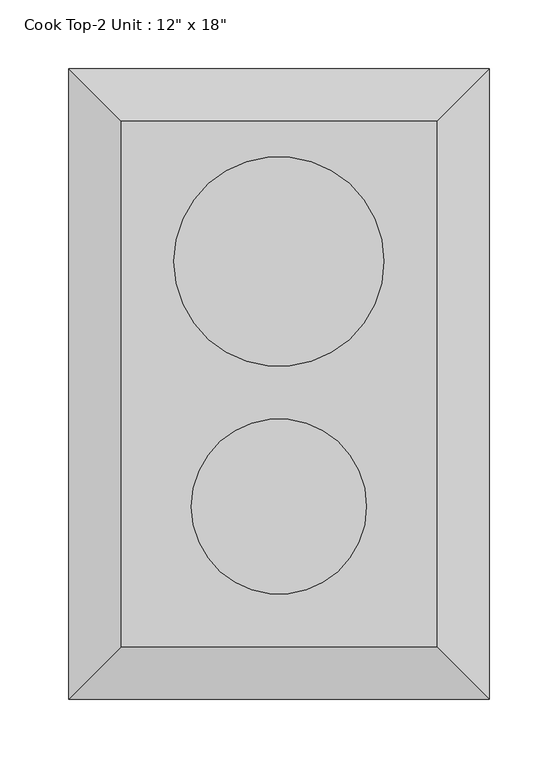
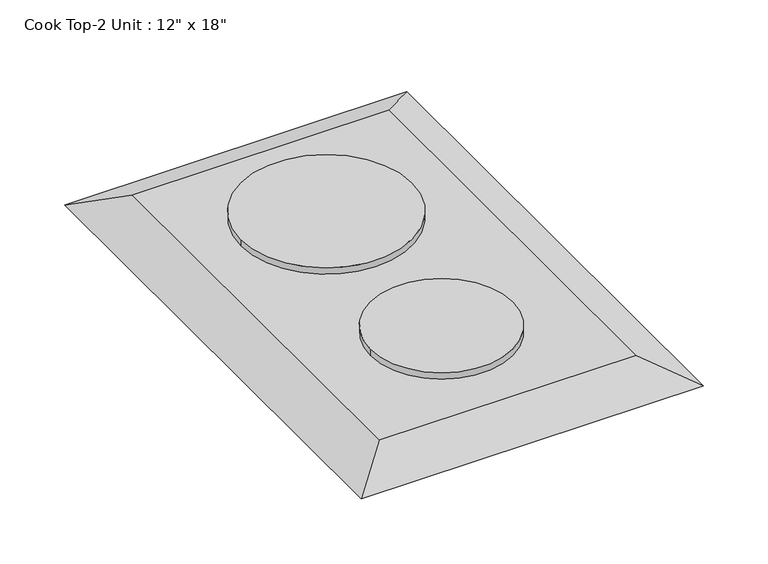
"""IFC4 building model written with IfcOpenShell, lengths in millimetres: proxy geometry."""

from ifc_helpers import new_model, si_unit, point, frame, frame_2d, origin, place, context, project, spatial, circle_curve, trimmed, segment, composite_curve, outline, extrude, faceted_brep, source, transform, mapped, element, save


def proxy_fb8a77b2(model_context):
    return source(origin(), model_context, "Body", "SolidModel", [
        faceted_brep([(190.5, 220.7247956, 933.45), (-38.1, 220.7247956, 933.45), (-38.1, -160.2752044, 933.45), (190.5, -160.2752044, 933.45), (228.6, 258.8247956, 914.4), (228.6, -198.3752044, 914.4), (-76.2, -198.3752044, 914.4), (-76.2, 258.8247956, 914.4)], [[[0, 1, 2, 3]], [[4, 5, 6, 7]], [[4, 7, 1, 0]], [[7, 6, 2, 1]], [[6, 5, 3, 2]], [[5, 4, 0, 3]]]),
        extrude(outline(composite_curve([segment(trimmed(circle_curve(frame_2d((76.2, 119.1247956)), 76.2), [point((152.4, 119.1247956))], [point((0.0, 119.1247956))], False, "CARTESIAN"), True, "CONTINUOUS"), segment(trimmed(circle_curve(frame_2d((76.2, 119.1247956)), 76.2), [point((0.0, 119.1247956))], [point((152.4, 119.1247956))], False, "CARTESIAN"), True, "CONTINUOUS")], self_intersect=False)), frame((0.0, 0.0, 933.45), z_axis=(0.0, 0.0, 1.0), x_axis=(1.0, 0.0, 0.0)), (0.0, 0.0, 1.0), 6.35),
        extrude(outline(composite_curve([segment(trimmed(circle_curve(frame_2d((76.2, -58.6752044)), 63.5), [point((139.7, -58.6752044))], [point((12.7, -58.6752044))], False, "CARTESIAN"), True, "CONTINUOUS"), segment(trimmed(circle_curve(frame_2d((76.2, -58.6752044)), 63.5), [point((12.7, -58.6752044))], [point((139.7, -58.6752044))], False, "CARTESIAN"), True, "CONTINUOUS")], self_intersect=False)), frame((0.0, 0.0, 933.45), z_axis=(0.0, 0.0, 1.0), x_axis=(1.0, 0.0, 0.0)), (0.0, 0.0, 1.0), 6.35),
    ])


if __name__ == "__main__":
    model = new_model("IFC4")
    model_context = context("Model", 3, world=origin())
    ifc_project = project(units=[si_unit("LENGTHUNIT", "METRE", prefix="MILLI")], contexts=[model_context])
    site = spatial("IfcSite", under=ifc_project)
    building = spatial("IfcBuilding", under=site)
    placement = place(None, origin())
    proxy_shape = proxy_fb8a77b2(model_context)
    element("IfcBuildingElementProxy", 1, Name="Cook Top-2 Unit : 12\" x 18\"", ObjectType="Cook Top-2 Unit : 12\" x 18\"", at=placement, inside=building, context=model_context, shape_type="MappedRepresentation", body=[
        mapped(proxy_shape, transform((0.0, 0.0, 0.0), x_axis=(1.0, 0.0, 0.0), y_axis=(0.0, 1.0, 0.0), z_axis=(0.0, 0.0, 1.0))),
    ])
    save(model, "model.ifc")

# Revit data of these elements
# Type "Cook Top-2 Unit : 12\" x 18\""
#   Assembly Code = "E1090400"
#   Counter Height = 3' - 0"
#   Depth = 1' - 6"
#   Width = 1' - 0"
#   Burner Material = Metal - Chrome
#   Cooktop Material = Metal - Steel, Polished
#   Default Elevation = 0
# Element 1 (IfcBuildingElementProxy, "Cook Top-2 Unit : 12\" x 18\"")
#   Materials on its faces: "Metal - Steel, Polished", "Metal - Chrome"
# Materials
#   "Metal - Chrome": colour RGB 17 17 17, transparency 0
#   "Metal - Steel, Polished": colour RGB 57 57 57, transparency 0
